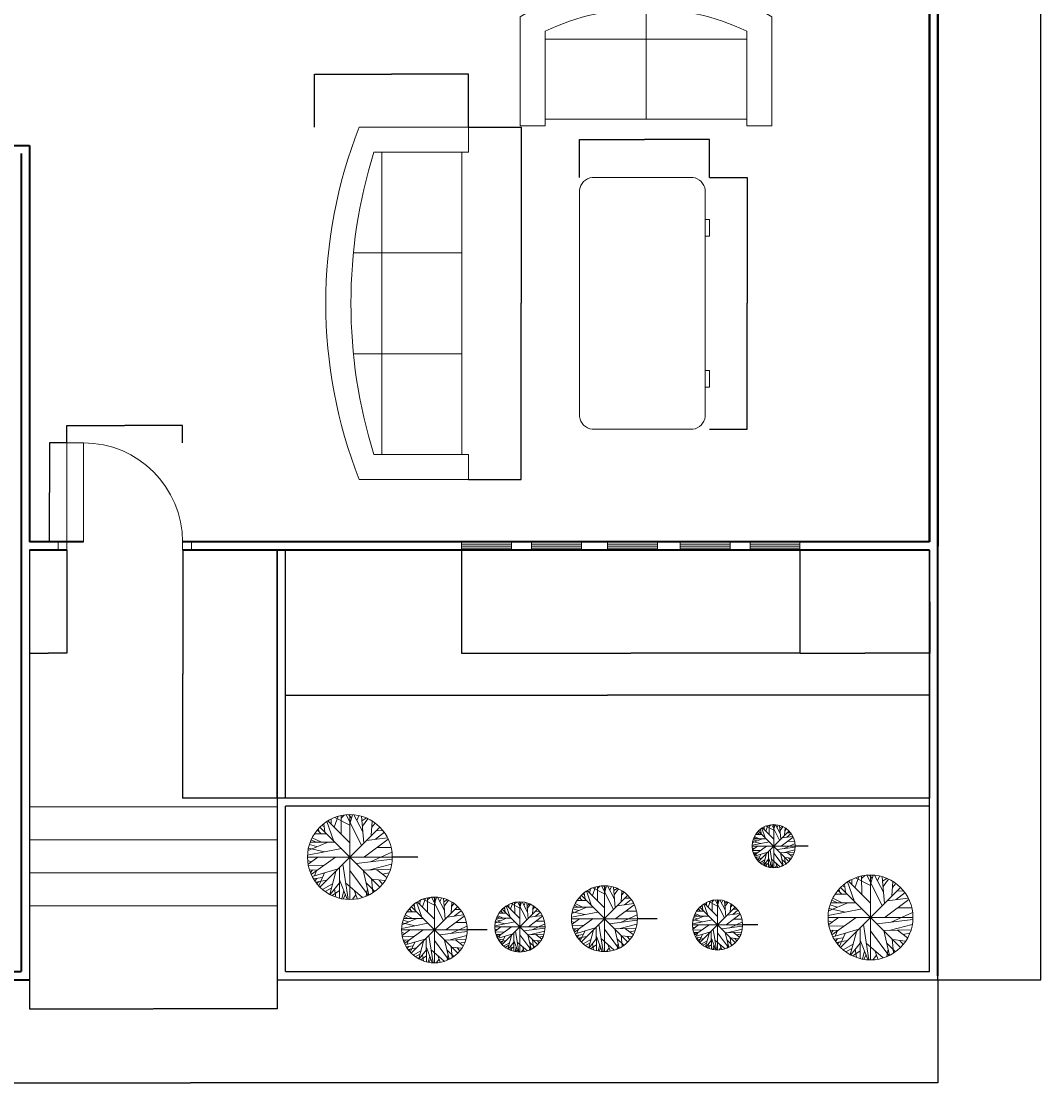
# Model space of a CAD drawing. Units: millimetres. Extents: x 1194 to 22780, y 83 to 13378.
# Tile 1 of 6: x 5317 to 11490, y 83 to 6507. Entities that reach past the tile are written whole.
import ezdxf

# ---------------------------------------------------------------- set-up
doc = ezdxf.new("R2010")
doc.units = ezdxf.units.MM
for name, color, linetype, lineweight in [('A-ANNO-DIMS', 2, 'Continuous', 18), ('A-DOOR', 3, 'Continuous', 18), ('A-FLOR-EDGE', 9, 'Continuous', 25), ('A-FLOR-STRS', 7, 'Continuous', 18), ('A-FURN', 8, 'Continuous', 18), ('A-GLAZ', 4, 'Continuous', 18), ('A-WALL', 7, 'Continuous', 35), ('L-PLNT', 3, 'Continuous', 13)]:
    doc.layers.add(name, color=color, linetype=linetype, lineweight=lineweight)
doc.styles.get("Standard").update_dxf_attribs({"font": 'arial.ttf'})
doc.dimstyles.get("Standard").update_dxf_attribs({"dimtxt": 0.18, "dimasz": 0.18, "dimexe": 0.18, "dimexo": 0.0625, "dimgap": 0.09, "dimtad": 0, "dimtih": 1, "dimtoh": 1, "dimdec": 4, "dimzin": 0, "dimdsep": 46, "dimtxsty": 'Standard', "dimcen": 0.09, "dimadec": 0, "dimazin": 0, "dimtfac": 1, "dimtdec": 4, "dimtofl": 0, "dimtmove": 0, "dimatfit": 3, "dimfxl": 1, "dimtolj": 1, "dimtzin": 0, "dimarcsym": 0})

# ---------------------------------------------------------------- blocks, each defined once
blk = doc.blocks.new('Sofa - Roundback 7 ft.')
for p, q in [((-12.00002, -32.44210000000393), (-12.00003, -6.597100000003898)), ((11.99996999999999, -32.44210000000393), (11.99997999999999, -6.597100000003898)), ((-36.000027, -34.00000000000395), (-36.000027, -11.46960000000396)), ((35.99997999999999, -34.00000000000395), (35.99997999999999, -11.46960000000396)), ((-35.999844, -13.38190000000397), (35.99979999999999, -13.38190000000397)), ((-36.000027, -32.44210000000393), (35.99997999999999, -32.44210000000393))]:
    blk.add_line(p, q)
for points in [[(-36.000027, -34.00000000000395), (-42.000027, -34.00000000000395), (-42.000027, -8.000000000003944)], [(41.99997999999999, -8.000000000003944), (41.99997999999999, -34.00000000000395), (35.99997999999999, -34.00000000000395)]]:
    blk.add_lwpolyline(points)
for centre, radius, start, end in [((0, -114.2500000000039), 114.2500000000039, 68.43141000000072, 111.5686000000006), ((-1.00000000032e-05, -127.1968000000039), 121.1967999999973, 72.72032999999948, 107.2797000000005)]:
    blk.add_arc(centre, radius, start, end)
blk = doc.blocks.new('Sofa - Roundback Loveseat 5 ft.')
for p, q in [((0, -32.44198000000246), (0, -5.999980000002448)), ((-23.99999999999999, -33.99998000000245), (-23.99999999999999, -11.46958000000243)), ((24.00004000000001, -33.99998000000245), (24.00004000000001, -11.46958000000243)), ((-23.99979999999998, -13.38178000000245), (23.99986, -13.38178000000245)), ((-23.99999999999999, -32.44198000000246), (24.00004000000001, -32.44198000000246))]:
    blk.add_line(p, q)
for points in [[(-23.99999999999999, -33.99998000000245), (-29.99999999999999, -33.99998000000245), (-29.99999999999999, -7.999980000002448)], [(30.00004000000001, -7.999980000002448), (30.00004000000001, -33.99998000000245), (24.00004000000001, -33.99998000000245)]]:
    blk.add_lwpolyline(points)
for centre, radius, start, end in [((0, -60.24998000000245), 60.24998000000245, 60.13715000000122, 119.862800000004), ((0, -61.38438000000245), 55.38444000000723, 64.32083000000306, 115.6791999999996)]:
    blk.add_arc(centre, radius, start, end)
blk = doc.blocks.new('Desk - 30 x 60 in.')
for p, q in [((-26.999995, 0), (26.999995, 0)), ((-29.999995, -27), (-29.999995, -3)), ((29.999995, -3), (29.999995, -27)), ((26.999995, -30), (-26.999995, -30)), ((-20.000005, -30), (-20.000005, -31)), ((-16.000005, -31), (-16.000005, -30)), ((15.999995, -31), (15.999995, -30)), ((19.999995, -30), (19.999995, -31)), ((-20.000005, -31), (-16.000005, -31)), ((19.999995, -31), (15.999995, -31))]:
    blk.add_line(p, q)
for centre, radius, start, end in [((-26.499995, -3.5), 3.535534000004229, 98.1300999999916, 171.8698999999352), ((26.499995, -3.5), 3.535533999997753, 8.130102000022115, 81.8698999999439), ((-26.499995, -26.5), 3.535534000000845, 188.1301000000653, 261.8699000000085), ((26.499995, -26.5), 3.535534000004826, 278.1301000000561, 351.8698999999439)]:
    blk.add_arc(centre, radius, start, end)
blk = doc.blocks.new('Window - Wood Frame 36 in. Wide plan')
for p, q in [((0, 6), (0, 0)), ((0, 4.5), (36, 4.5)), ((0, 3), (36, 3)), ((0, 1.5), (36, 1.5)), ((36, 6), (36, 0))]:
    blk.add_line(p, q)
blk = doc.blocks.new('Tree - deciduous plan')
for p, q in [((-37.01069999999993, 47.04079999999987), (-35.25, 35.52979999999991)), ((-32.60919999999999, 50.42639999999995), (-23.27819999999997, 23.56739999999991)), ((-31.20079999999996, 51.10349999999994), (-0.2148999999999432, 20.18179999999984)), ((-26.44719999999995, 46.58939999999984), (-26.27120000000002, 53.81159999999988)), ((-22.04579999999999, 42.07529999999986), (-16.58809999999994, 57.64859999999988)), ((-21.16559999999993, 55.84359999999981), (-0.0387999999999238, 45.00939999999991)), ((-12.53879999999992, 54.94059999999979), (-7.961299999999937, 59.45459999999991)), ((-12.36270000000002, 32.14429999999993), (-12.53879999999992, 58.77760000000001)), ((-5.320499999999924, 59.68059999999979), (16.51049999999998, 16.79629999999986)), ((2.426000000000044, 54.94059999999979), (-1.447199999999952, 59.90559999999982)), ((0, 59.99959999999987), (0, -60.00000000000011)), ((0.4894000000000461, 48.62079999999991), (3.658400000000028, 59.68059999999979)), ((18.27110000000004, 35.52979999999991), (5.418999999999982, 59.68059999999979)), ((9.820299999999975, 51.55489999999986), (12.81330000000002, 58.55159999999989)), ((19.67950000000007, 19.50469999999984), (16.33440000000007, 57.64859999999988)), ((17.03870000000006, 51.10349999999994), (23.20060000000001, 55.16659999999991)), ((17.74290000000007, 43.65519999999992), (25.48940000000005, 54.26359999999988)), ((31.65129999999999, 50.87779999999987), (30.24290000000008, 30.56429999999989)), ((31.1232, 42.52669999999989), (35.87670000000003, 48.16929999999991)), ((-49.86270000000001, 32.82139999999993), (-32.78530000000001, 32.82139999999993)), ((-45.81339999999999, 38.23829999999987), (-40.53179999999997, 33.04709999999989)), ((-43.8768, 36.43259999999998), (-44.40499999999997, 40.26959999999997)), ((42, 41.99999999999988), (-42, -42.00000000000011)), ((42, -42.00000000000011), (-42, 41.99999999999988)), ((-40.17970000000002, 44.55799999999988), (-36.48249999999996, 43.20379999999988)), ((36.22879999999998, 25.14739999999995), (48.90489999999999, 35.07839999999987)), ((37.10910000000001, 37.10979999999995), (46.61609999999996, 37.56119999999987)), ((-32.25709999999992, 20.63329999999985), (-59.19370000000004, 9.347999999999843)), ((-57.08100000000001, 17.92479999999989), (-47.04579999999999, 14.7648999999999)), ((-56.02469999999994, 20.85899999999992), (-20.8134, 20.85899999999992)), ((-54.79229999999995, 24.47019999999986), (-47.75, 21.08469999999988)), ((-53.20780000000002, 27.4043999999999), (-40.17970000000002, 20.85899999999992)), ((54.36260000000004, 25.37309999999991), (20.91190000000006, 0.3197999999998728)), ((23.37670000000003, 23.34169999999994), (53.30629999999996, 27.4043999999999)), ((-59.72190000000001, 2.802499999999895), (-12.01059999999995, 12.05649999999991)), ((-58.66559999999992, 12.73359999999991), (-35.95429999999999, 7.542399999999929)), ((-54.61619999999993, -24.73350000000016), (-20.28530000000001, 0.0940999999999122)), ((29.36260000000004, -6.677100000000109), (59.46820000000002, 7.090999999999894)), ((38.51750000000004, 13.4106999999999), (58.23590000000002, 13.63639999999987)), ((-60, -1.137e-13), (60, -1.137e-13)), ((-59.72190000000001, -4.871400000000107), (-54.26409999999998, -6.677100000000109)), ((-45.2853, -0.1316000000001622), (-59.01769999999999, -10.06270000000006)), ((-58.48950000000002, -12.31970000000012), (-36.48249999999996, -11.64260000000013)), ((-10.07399999999995, -10.06270000000006), (-2.503600000000005, -59.71780000000013)), ((9.29219999999998, -9.159800000000132), (59.64430000000004, -2.84010000000012)), ((26.36969999999997, -18.41380000000015), (58.94010000000003, -9.836900000000128)), ((-57.08100000000001, -18.41380000000015), (-45.2853, -17.9624)), ((-52.67970000000002, -18.1880000000001), (-55.49659999999994, -22.02510000000007)), ((-53.20780000000002, -27.44200000000012), (-16.76409999999998, -16.60810000000015)), ((-38.94719999999995, -29.02190000000008), (-51.44719999999995, -30.60180000000014)), ((-47.2219, -19.31660000000011), (-50.21479999999996, -26.31350000000009)), ((-35.95429999999999, -22.4765000000001), (-44.05290000000002, -40.53290000000015)), ((-19.93309999999997, -20.21940000000018), (-28.55989999999997, -52.72100000000012)), ((-14.82749999999998, -15.02820000000008), (-14.65149999999994, -57.68650000000014)), ((-0.0387999999999238, -19.09090000000015), (25.8415, -53.84950000000015)), ((18.6232, -18.63940000000013), (26.72180000000003, -53.39810000000011)), ((18.79920000000004, -18.63940000000013), (57.35559999999998, -17.28530000000012)), ((38.16539999999998, -18.1880000000001), (52.42600000000004, -29.02190000000008)), ((45.91190000000006, -24.05640000000017), (55.59500000000003, -22.25080000000014)), ((-46.51769999999999, -30.15040000000011), (-49.51059999999995, -33.53600000000006)), ((-32.43309999999997, -32.40750000000014), (-48.10209999999995, -35.56740000000002)), ((-43.70079999999996, -34.66450000000009), (-46.69370000000003, -37.37300000000016)), ((-24.68669999999998, -37.8244000000002), (-38.77120000000002, -45.72410000000013)), ((-26.27120000000002, -43.91850000000011), (-34.72190000000001, -48.65830000000006)), ((-14.65149999999994, -36.24450000000013), (-27.67970000000003, -52.94670000000007)), ((-14.65149999999994, -32.18180000000007), (-3.912000000000034, -59.49220000000014)), ((-6.200799999999958, -36.24450000000013), (17.91899999999998, -57.00940000000014)), ((22.84850000000006, -36.47020000000009), (35.34850000000006, -48.43260000000009)), ((24.78520000000003, -44.82130000000006), (23.02459999999996, -54.97800000000006)), ((30.41899999999998, -30.15040000000011), (32.35559999999998, -50.01250000000016)), ((31.47530000000006, -31.27900000000011), (49.60910000000001, -33.3103000000001)), ((41.51049999999997, -32.6332000000001), (46.08799999999996, -38.05010000000016)), ((-14.65149999999994, -47.30410000000006), (-25.03879999999993, -54.30090000000006)), ((-21.51769999999999, -45.49840000000005), (-19.93309999999997, -56.1065000000001)), ((-8.48950000000002, -47.52980000000014), (-11.48249999999996, -58.58930000000009)), ((-6.376800000000002, -52.72100000000012), (-9.369799999999941, -58.81500000000006)), ((8.41190000000006, -53.17240000000004), (3.834400000000073, -59.49220000000014)), ((5.947099999999977, -46.62690000000009), (10.52459999999996, -58.58930000000009))]:
    blk.add_line(p, q)
blk.add_circle((0, -1.137e-13), 60)
blk = doc.blocks.new('DOOR-SWING-600')
for p, q in [((-0.0004640084134735, -0.0001152583831754), (-0.0004640084134735, 599.9998847416168)), ((-0.0004640084134735, 599.9998847416168), (99.99953599158653, 599.9998847416168)), ((99.99953599158653, 599.9998847416168), (99.99953599158653, -0.0001152583831754))]:
    blk.add_line(p, q)
blk.add_arc((99.99953599158653, -0.0001152583831754), 600, 0, 90)
blk = doc.blocks.new('*D19')
at = {"layer": 'A-ANNO-DIMS', "color": 0, "lineweight": -2, "transparency": 16777216}
for p, q in [((5594.319535991585, 3955.836384741617), (5594.319535991585, 4060.953884741617)), ((5594.499535991586, 4060.773884741617), (5943.313881148475, 4060.773884741617)), ((6294.139535991585, 4060.773884741617), (5945.325190834696, 4060.773884741617)), ((6294.319535991586, 3955.836384741617), (6294.319535991586, 4060.953884741617))]:
    blk.add_line(p, q, dxfattribs=at)
at = {"layer": 'A-ANNO-DIMS', "color": 0, "transparency": 16777216}
for points in [[(5594.499535991586, 4060.803884741616), (5594.499535991586, 4060.743884741617), (5594.319535991585, 4060.773884741617)], [(6294.139535991585, 4060.803884741616), (6294.139535991585, 4060.743884741617), (6294.319535991586, 4060.773884741617)]]:
    blk.add_solid(points, dxfattribs=at)
at = {"layer": 'Defpoints', "color": 0, "transparency": 16777216}
for p in [(6294.319535991586, 4060.773884741617), (5594.319535991585, 3955.773884741617), (6294.319535991586, 3955.773884741617)]:
    blk.add_point(p, dxfattribs=at)
at = {"layer": 'A-ANNO-DIMS', "color": 0, "transparency": 16777216, "insert": (5944.319535991585, 4060.773884741617), "char_height": 0.18, "attachment_point": 5}
blk.add_mtext('\\A1;DOOR 700 TYP.', dxfattribs=at)
blk = doc.blocks.new('*D20')
at = {"layer": 'A-ANNO-DIMS', "color": 0, "lineweight": -2, "transparency": 16777216}
for p, q in [((5594.257035991587, 3955.773884741619), (5489.139535991589, 3955.773884741619)), ((5489.319535991589, 3955.593884741619), (5489.319535991589, 3655.955787879409)), ((5489.319535991589, 3355.953884741619), (5489.319535991589, 3655.591981603829)), ((5594.257035991587, 3355.773884741619), (5489.139535991589, 3355.773884741619))]:
    blk.add_line(p, q, dxfattribs=at)
at = {"layer": 'A-ANNO-DIMS', "color": 0, "transparency": 16777216}
for points in [[(5489.289535991589, 3955.593884741619), (5489.349535991589, 3955.593884741619), (5489.319535991589, 3955.773884741619)], [(5489.289535991589, 3355.953884741619), (5489.349535991589, 3355.953884741619), (5489.319535991589, 3355.773884741619)]]:
    blk.add_solid(points, dxfattribs=at)
at = {"layer": 'Defpoints', "color": 0, "transparency": 16777216}
for p in [(5489.319535991589, 3955.773884741619), (5594.319535991587, 3955.773884741619), (5594.319535991587, 3355.773884741619)]:
    blk.add_point(p, dxfattribs=at)
at = {"layer": 'A-ANNO-DIMS', "color": 0, "transparency": 16777216, "insert": (5489.319535991589, 3655.773884741616), "char_height": 0.18, "attachment_point": 5}
blk.add_mtext('\\A1;600 TYP.', dxfattribs=at)
blk = doc.blocks.new('*D31')
at = {"layer": 'A-ANNO-DIMS', "color": 0, "lineweight": -2, "transparency": 16777216}
for p, q in [((8024.9386296235, 5866.896359479268), (8345.096343171488, 5866.896359479268)), ((8344.91634317149, 5866.716359479267), (8344.91634317149, 4800.279344007587)), ((8344.91634317149, 3733.475943815578), (8344.91634317149, 4799.912959287258)), ((8024.93893202036, 3733.295943815578), (8345.096343171488, 3733.295943815578))]:
    blk.add_line(p, q, dxfattribs=at)
at = {"layer": 'A-ANNO-DIMS', "color": 0, "transparency": 16777216}
for points in [[(8344.886343171485, 5866.716359479267), (8344.946343171488, 5866.716359479267), (8344.91634317149, 5866.896359479268)], [(8344.88634317149, 3733.475943815578), (8344.94634317149, 3733.475943815578), (8344.91634317149, 3733.295943815578)]]:
    blk.add_solid(points, dxfattribs=at)
at = {"layer": 'Defpoints', "color": 0, "transparency": 16777216}
for p in [(8024.8761296235, 5866.896359479268), (8344.91634317149, 5866.896359479268), (8024.876432020361, 3733.295943815578)]:
    blk.add_point(p, dxfattribs=at)
at = {"layer": 'A-ANNO-DIMS', "color": 0, "transparency": 16777216, "insert": (8344.91634317149, 4800.096151647419), "char_height": 0.18, "attachment_point": 5}
blk.add_mtext('\\A1;SOFA 2134 TYP.', dxfattribs=at)
blk = doc.blocks.new('*D32')
at = {"layer": 'A-ANNO-DIMS', "color": 0, "lineweight": -2, "transparency": 16777216}
for p, q in [((7093.54276755999, 5866.958727480659), (7093.542722183807, 6187.116289830213)), ((7093.722722209318, 6186.936289855724), (7558.611388229824, 6186.936355744759)), ((8024.69608426397, 6186.936421803308), (7559.807418243467, 6186.936355914273)), ((8024.876129614641, 5866.958859479268), (8024.876084238458, 6187.116421828821))]:
    blk.add_line(p, q, dxfattribs=at)
at = {"layer": 'A-ANNO-DIMS', "color": 0, "transparency": 16777216}
for points in [[(7093.722722205066, 6186.966289855724), (7093.72272221357, 6186.906289855723), (7093.542722209318, 6186.936289830213)], [(8024.696084259717, 6186.966421803308), (8024.696084268221, 6186.906421803308), (8024.87608426397, 6186.93642182882)]]:
    blk.add_solid(points, dxfattribs=at)
at = {"layer": 'Defpoints', "color": 0, "transparency": 16777216}
for p in [(7093.542722209318, 6186.936289830213), (7093.542767568848, 5866.896227480658), (8024.876129623498, 5866.896359479268)]:
    blk.add_point(p, dxfattribs=at)
at = {"layer": 'A-ANNO-DIMS', "color": 0, "transparency": 16777216, "insert": (7559.209403236645, 6186.936355829516), "char_height": 0.18, "attachment_point": 5}
blk.add_mtext('\\A1;931 TYP.', dxfattribs=at)
blk = doc.blocks.new('*D43')
at = {"layer": 'A-ANNO-DIMS', "color": 0, "lineweight": -2, "transparency": 16777216}
for p, q in [((9484.758350555348, 5562.096129861136), (9713.475813321516, 5562.096129861136)), ((9713.295813321516, 5561.916129861136), (9713.295813321516, 4800.279323551006)), ((9713.29581332152, 4038.276378086716), (9713.295813321516, 4799.913184396845)), ((9484.758350555348, 4038.096378086716), (9713.475813321518, 4038.096378086716))]:
    blk.add_line(p, q, dxfattribs=at)
at = {"layer": 'A-ANNO-DIMS', "color": 0, "transparency": 16777216}
for points in [[(9713.265813321515, 5561.916129861136), (9713.325813321517, 5561.916129861136), (9713.295813321516, 5562.096129861136)], [(9713.265813321517, 4038.276378086716), (9713.325813321519, 4038.276378086716), (9713.29581332152, 4038.096378086716)]]:
    blk.add_solid(points, dxfattribs=at)
at = {"layer": 'Defpoints', "color": 0, "transparency": 16777216}
for p in [(9484.695850555348, 5562.096129861136), (9713.295813321516, 5562.096129861136), (9484.695850555348, 4038.096378086716)]:
    blk.add_point(p, dxfattribs=at)
at = {"layer": 'A-ANNO-DIMS', "color": 0, "transparency": 16777216, "insert": (9713.295813321516, 4800.096253973922), "char_height": 0.18, "attachment_point": 5}
blk.add_mtext('\\A1;DESK 1524', dxfattribs=at)
blk = doc.blocks.new('*D44')
at = {"layer": 'A-ANNO-DIMS', "color": 0, "lineweight": -2, "transparency": 16777216}
for p, q in [((8697.295847668129, 5562.158629861134), (8697.295847668129, 5790.876092627298)), ((8697.475847668127, 5790.696092627298), (9090.707738606961, 5790.696092627298)), ((9484.515850555345, 5790.696092627298), (9091.283959616509, 5790.696092627298)), ((9484.695850555345, 5562.158629861134), (9484.695850555345, 5790.876092627298))]:
    blk.add_line(p, q, dxfattribs=at)
at = {"layer": 'A-ANNO-DIMS', "color": 0, "transparency": 16777216}
for points in [[(8697.475847668127, 5790.726092627298), (8697.475847668127, 5790.666092627298), (8697.295847668129, 5790.696092627298)], [(9484.515850555345, 5790.726092627298), (9484.515850555345, 5790.666092627298), (9484.695850555345, 5790.696092627298)]]:
    blk.add_solid(points, dxfattribs=at)
at = {"layer": 'Defpoints', "color": 0, "transparency": 16777216}
for p in [(8697.295847668129, 5790.696092627298), (8697.295847668129, 5562.096129861135), (9484.695850555345, 5562.096129861135)]:
    blk.add_point(p, dxfattribs=at)
at = {"layer": 'A-ANNO-DIMS', "color": 0, "transparency": 16777216, "insert": (9090.995849111736, 5790.696092627298), "char_height": 0.18, "attachment_point": 5}
blk.add_mtext('\\A1;787', dxfattribs=at)
blk = doc.blocks.new('*D51')
at = {"layer": 'A-ANNO-DIMS', "color": 0, "lineweight": -2, "transparency": 16777216}
for p, q in [((1817.4811, 705.711385), (1817.4811, 83.093885)), ((10867.4811, 705.711385), (10867.4811, 83.093885)), ((1817.6611, 83.273885), (6342.122634788541, 83.273885)), ((10867.3011, 83.273885), (6342.839565211459, 83.273885))]:
    blk.add_line(p, q, dxfattribs=at)
at = {"layer": 'A-ANNO-DIMS', "color": 0, "transparency": 16777216}
for points in [[(1817.6611, 83.30388500000001), (1817.6611, 83.243885), (1817.4811, 83.273885)], [(10867.3011, 83.30388500000001), (10867.3011, 83.243885), (10867.4811, 83.273885)]]:
    blk.add_solid(points, dxfattribs=at)
at = {"layer": 'Defpoints', "color": 0, "transparency": 16777216}
for p in [(1817.4811, 705.773885), (10867.4811, 705.773885), (10867.4811, 83.273885)]:
    blk.add_point(p, dxfattribs=at)
at = {"layer": 'A-ANNO-DIMS', "color": 0, "transparency": 16777216, "insert": (6342.4811, 83.273885), "char_height": 0.18, "attachment_point": 5}
blk.add_mtext('\\A1;9050', dxfattribs=at)
blk = doc.blocks.new('*D52')
at = {"layer": 'A-ANNO-DIMS', "color": 0, "lineweight": -2, "transparency": 16777216}
for p, q in [((10867.5436, 12755.77388500001), (11490.1611, 12755.77388500001)), ((11489.9811, 12755.593885), (11489.98110000001, 6730.955788137794)), ((11489.98110000001, 705.9538850000002), (11489.98110000001, 6730.591981862215)), ((10867.5436, 705.7738850000001), (11490.16110000001, 705.7738850000003))]:
    blk.add_line(p, q, dxfattribs=at)
at = {"layer": 'A-ANNO-DIMS', "color": 0, "transparency": 16777216}
for points in [[(11489.9511, 12755.593885), (11490.01110000001, 12755.593885), (11489.9811, 12755.77388500001)], [(11489.95110000001, 705.9538850000002), (11490.01110000001, 705.9538850000002), (11489.98110000001, 705.7738850000003)]]:
    blk.add_solid(points, dxfattribs=at)
at = {"layer": 'Defpoints', "color": 0, "transparency": 16777216}
for p in [(10867.4811, 12755.77388500001), (11489.9811, 12755.77388500001), (10867.4811, 705.7738850000001)]:
    blk.add_point(p, dxfattribs=at)
at = {"layer": 'A-ANNO-DIMS', "color": 0, "transparency": 16777216, "insert": (11489.98110000001, 6730.773884999999), "char_height": 0.18, "attachment_point": 5}
blk.add_mtext('\\A1;12050', dxfattribs=at)
blk = doc.blocks.new('*D57')
at = {"layer": 'A-ANNO-DIMS', "color": 0, "lineweight": -2, "transparency": 16777216}
for p, q in [((5367.4811, 1152.796637), (5367.4811, 530.1791370000001)), ((6867.4811, 1152.796637), (6867.4811, 530.1791370000001)), ((5367.6611, 530.359137), (6117.131106821283, 530.359137)), ((6867.3011, 530.359137), (6117.831093178717, 530.359137))]:
    blk.add_line(p, q, dxfattribs=at)
at = {"layer": 'A-ANNO-DIMS', "color": 0, "transparency": 16777216}
for points in [[(5367.6611, 530.389137), (5367.6611, 530.3291370000001), (5367.4811, 530.359137)], [(6867.3011, 530.389137), (6867.3011, 530.3291370000001), (6867.4811, 530.359137)]]:
    blk.add_solid(points, dxfattribs=at)
at = {"layer": 'Defpoints', "color": 0, "transparency": 16777216}
for p in [(5367.4811, 1152.859137), (6867.4811, 1152.859137), (5367.4811, 530.359137)]:
    blk.add_point(p, dxfattribs=at)
at = {"layer": 'A-ANNO-DIMS', "color": 0, "transparency": 16777216, "insert": (6117.4811, 530.359137), "char_height": 0.18, "attachment_point": 5}
blk.add_mtext('\\A1;1500', dxfattribs=at)
blk = doc.blocks.new('*D58')
at = {"layer": 'A-ANNO-DIMS', "color": 0, "lineweight": -2, "transparency": 16777216}
for p, q in [((6917.4811, 1805.836385), (6917.4811, 2428.453885)), ((6917.661100000001, 2428.273885), (8867.122696180082, 2428.273885)), ((10817.3011, 2428.273885), (8867.83950381992, 2428.273885)), ((10817.4811, 1805.836385), (10817.4811, 2428.453885))]:
    blk.add_line(p, q, dxfattribs=at)
at = {"layer": 'A-ANNO-DIMS', "color": 0, "transparency": 16777216}
for points in [[(6917.661100000001, 2428.303885), (6917.661100000001, 2428.243885), (6917.4811, 2428.273885)], [(10817.3011, 2428.303885), (10817.3011, 2428.243885), (10817.4811, 2428.273885)]]:
    blk.add_solid(points, dxfattribs=at)
at = {"layer": 'Defpoints', "color": 0, "transparency": 16777216}
for p in [(10817.4811, 2428.273885), (6917.4811, 1805.773885), (10817.4811, 1805.773885)]:
    blk.add_point(p, dxfattribs=at)
at = {"layer": 'A-ANNO-DIMS', "color": 0, "transparency": 16777216, "insert": (8867.4811, 2428.273885), "char_height": 0.18, "attachment_point": 5}
blk.add_mtext('\\A1;3900', dxfattribs=at)
blk = doc.blocks.new('*D62')
at = {"layer": 'A-ANNO-DIMS', "color": 0, "lineweight": -2, "transparency": 16777216}
for p, q in [((6917.418600000003, 3305.773885000002), (6294.801100000007, 3305.773885000002)), ((6294.981100000008, 3305.593885000002), (6294.981100000008, 2555.955788137791)), ((6294.981100000008, 1805.953885000001), (6294.981100000008, 2555.591981862212)), ((6917.418600000003, 1805.773885000001), (6294.801100000007, 1805.773885))]:
    blk.add_line(p, q, dxfattribs=at)
at = {"layer": 'A-ANNO-DIMS', "color": 0, "transparency": 16777216}
for points in [[(6294.951100000008, 3305.593885000002), (6295.011100000007, 3305.593885000002), (6294.981100000008, 3305.773885000002)], [(6294.951100000009, 1805.953885000001), (6295.011100000007, 1805.953885000001), (6294.981100000008, 1805.773885)]]:
    blk.add_solid(points, dxfattribs=at)
at = {"layer": 'Defpoints', "color": 0, "transparency": 16777216}
for p in [(6294.981100000008, 3305.773885000002), (6917.481100000003, 3305.773885000002), (6917.481100000003, 1805.773885000001)]:
    blk.add_point(p, dxfattribs=at)
at = {"layer": 'A-ANNO-DIMS', "color": 0, "transparency": 16777216, "insert": (6294.981100000007, 2555.773884999999), "char_height": 0.18, "attachment_point": 5}
blk.add_mtext('\\A1;1500', dxfattribs=at)
blk = doc.blocks.new('*D67')
at = {"layer": 'A-ANNO-DIMS', "color": 0, "lineweight": -2, "transparency": 16777216}
for p, q in [((7983.786704999999, 3305.383366), (7983.786704999999, 2682.765866)), ((10032.104138, 3305.383366), (10032.104138, 2682.765866)), ((7983.966705, 2682.945866), (9007.480257789222, 2682.945866)), ((10031.924138, 2682.945866), (9008.410585210779, 2682.945866))]:
    blk.add_line(p, q, dxfattribs=at)
at = {"layer": 'A-ANNO-DIMS', "color": 0, "transparency": 16777216}
for points in [[(7983.966705, 2682.975866), (7983.966705, 2682.915866), (7983.786704999999, 2682.945866)], [(10031.924138, 2682.975866), (10031.924138, 2682.915866), (10032.104138, 2682.945866)]]:
    blk.add_solid(points, dxfattribs=at)
at = {"layer": 'Defpoints', "color": 0, "transparency": 16777216}
for p in [(7983.786704999999, 3305.445866), (10032.104138, 3305.445866), (7983.786704999999, 2682.945866)]:
    blk.add_point(p, dxfattribs=at)
at = {"layer": 'A-ANNO-DIMS', "color": 0, "transparency": 16777216, "insert": (9007.945421500002, 2682.945866), "char_height": 0.18, "attachment_point": 5}
blk.add_mtext('\\A1;2048.3', dxfattribs=at)
blk = doc.blocks.new('*D68')
at = {"layer": 'A-ANNO-DIMS', "color": 0, "lineweight": -2, "transparency": 16777216}
for p, q in [((10032.10416410359, 3305.383366005452), (10032.3642049862, 2682.765920703064)), ((10817.4811261036, 3305.711385005452), (10817.74116698636, 2683.093939328176)), ((10032.54412979215, 2682.945995865719), (10424.66001189933, 2683.109766028019)), ((10817.56109182371, 2683.273864134122), (10425.44520971652, 2683.110093971823))]:
    blk.add_line(p, q, dxfattribs=at)
at = {"layer": 'A-ANNO-DIMS', "color": 0, "transparency": 16777216}
for points in [[(10032.54411726242, 2682.975995863102), (10032.54414232187, 2682.915995868335), (10032.36412980785, 2682.945920687365)], [(10817.56107929398, 2683.303864131506), (10817.56110435343, 2683.243864136739), (10817.74109180801, 2683.273939312477)]]:
    blk.add_solid(points, dxfattribs=at)
at = {"layer": 'Defpoints', "color": 0, "transparency": 16777216}
for p in [(10032.104138, 3305.445866000001), (10817.4811, 3305.773885000001), (10032.36412980785, 2682.945920687365)]:
    blk.add_point(p, dxfattribs=at)
at = {"layer": 'A-ANNO-DIMS', "color": 0, "transparency": 16777216, "insert": (10425.05261080792, 2683.109929999921), "char_height": 0.18, "attachment_point": 5}
blk.add_mtext('\\A1;785.4', dxfattribs=at)
blk = doc.blocks.new('*D69')
at = {"layer": 'A-ANNO-DIMS', "color": 0, "lineweight": -2, "transparency": 16777216}
for p, q in [((5367.4811, 3305.711385), (5367.4811, 2683.093885)), ((5594.319536, 3305.711385), (5594.319536, 2683.093885)), ((5367.6611, 2683.273885), (5480.435522638472, 2683.273885)), ((5594.139536, 2683.273885), (5481.365113361528, 2683.273885))]:
    blk.add_line(p, q, dxfattribs=at)
at = {"layer": 'A-ANNO-DIMS', "color": 0, "transparency": 16777216}
for points in [[(5367.6611, 2683.303885000001), (5367.6611, 2683.243885), (5367.4811, 2683.273885)], [(5594.139536, 2683.303885000001), (5594.139536, 2683.243885), (5594.319536, 2683.273885)]]:
    blk.add_solid(points, dxfattribs=at)
at = {"layer": 'Defpoints', "color": 0, "transparency": 16777216}
for p in [(5367.4811, 3305.773885), (5594.319536, 3305.773885), (5367.4811, 2683.273885)]:
    blk.add_point(p, dxfattribs=at)
at = {"layer": 'A-ANNO-DIMS', "color": 0, "transparency": 16777216, "insert": (5480.900317999999, 2683.273885), "char_height": 0.18, "attachment_point": 5}
blk.add_mtext('\\A1;226.84', dxfattribs=at)
blk = doc.blocks.new('*D94')
at = {"layer": 'A-ANNO-DIMS', "color": 0, "lineweight": -2, "transparency": 16777216}
for p, q in [((7307.195641999998, 1448.826718), (7307.375642, 1448.826717999999)), ((7307.285641999998, 1448.736718), (7307.285641999998, 1448.916717999999)), ((7718.239941199906, 1448.8271692), (7564.312078999998, 1448.827000197628))]:
    blk.add_line(p, q, dxfattribs=at)
at = {"layer": 'A-ANNO-DIMS', "color": 0, "transparency": 16777216}
blk.add_solid([(7564.312078967062, 1448.857000197628), (7564.312079032936, 1448.797000197628), (7564.132078999998, 1448.827)], dxfattribs=at)
at = {"layer": 'Defpoints', "color": 0, "transparency": 16777216}
for p in [(7050.439205, 1448.826436), (7564.132078999998, 1448.827)]:
    blk.add_point(p, dxfattribs=at)
at = {"layer": 'A-ANNO-DIMS', "color": 0, "transparency": 16777216, "insert": (7718.921694269482, 1448.8271692), "char_height": 0.18, "attachment_point": 5}
blk.add_mtext('\\A1;2X ∅513.7', dxfattribs=at)
blk = doc.blocks.new('*D95')
at = {"layer": 'A-ANNO-DIMS', "color": 0, "lineweight": -2, "transparency": 16777216}
for p, q in [((8848.506493, 1076.128227999999), (8848.686492999996, 1076.128227999999)), ((8848.596493, 1076.038228), (8848.596493, 1076.218227999999)), ((9167.969441799922, 1076.127863199999), (9048.384586, 1076.127999794396))]:
    blk.add_line(p, q, dxfattribs=at)
at = {"layer": 'A-ANNO-DIMS', "color": 0, "transparency": 16777216}
blk.add_solid([(9048.384586034268, 1076.157999794396), (9048.384585965732, 1076.097999794396), (9048.204586, 1076.127999999999)], dxfattribs=at)
at = {"layer": 'Defpoints', "color": 0, "transparency": 16777216}
for p in [(8648.988399999995, 1076.128455999999), (9048.204586, 1076.127999999999)]:
    blk.add_point(p, dxfattribs=at)
at = {"layer": 'A-ANNO-DIMS', "color": 0, "transparency": 16777216, "insert": (9168.460144392013, 1076.127863199999), "char_height": 0.18, "attachment_point": 5}
blk.add_mtext('\\A1;∅399.2', dxfattribs=at)
blk = doc.blocks.new('*D96')
at = {"layer": 'A-ANNO-DIMS', "color": 0, "lineweight": -2, "transparency": 16777216}
for p, q in [((7819.127702999998, 1007.942615), (7819.307702999999, 1007.942615)), ((7819.217702999999, 1007.852615), (7819.217702999999, 1008.032615)), ((8137.805598999776, 1007.943231), (8018.515138000001, 1007.943000348035))]:
    blk.add_line(p, q, dxfattribs=at)
at = {"layer": 'A-ANNO-DIMS', "color": 0, "transparency": 16777216}
blk.add_solid([(8018.515137941994, 1007.973000348036), (8018.515138058008, 1007.913000348036), (8018.335138000001, 1007.943)], dxfattribs=at)
at = {"layer": 'Defpoints', "color": 0, "transparency": 16777216}
for p in [(7620.100267999998, 1007.94223), (8018.335138000001, 1007.943)]:
    blk.add_point(p, dxfattribs=at)
at = {"layer": 'A-ANNO-DIMS', "color": 0, "transparency": 16777216, "insert": (8138.296301591863, 1007.943231), "char_height": 0.18, "attachment_point": 5}
blk.add_mtext('\\A1;∅398.2', dxfattribs=at)
blk = doc.blocks.new('*D97')
at = {"layer": 'A-ANNO-DIMS', "color": 0, "lineweight": -2, "transparency": 16777216}
for p, q in [((9533.006967999992, 1038.522900999999), (9533.186967999996, 1038.522900999999)), ((9533.096967999993, 1038.432900999999), (9533.096967999996, 1038.612900999999)), ((9776.606814399982, 1038.523059399999), (9685.470621999995, 1038.523000117087))]:
    blk.add_line(p, q, dxfattribs=at)
at = {"layer": 'A-ANNO-DIMS', "color": 0, "transparency": 16777216}
blk.add_solid([(9685.470621980481, 1038.553000117087), (9685.470622019511, 1038.493000117087), (9685.290621999997, 1038.522999999999)], dxfattribs=at)
at = {"layer": 'Defpoints', "color": 0, "transparency": 16777216}
for p in [(9380.903314, 1038.522801999999), (9685.290621999997, 1038.522999999999)]:
    blk.add_point(p, dxfattribs=at)
at = {"layer": 'A-ANNO-DIMS', "color": 0, "transparency": 16777216, "insert": (9777.288199120308, 1038.523059399999), "char_height": 0.18, "attachment_point": 5}
blk.add_mtext('\\A1;2X ∅304.4', dxfattribs=at)
blk = doc.blocks.new('*D98')
at = {"layer": 'A-ANNO-DIMS', "color": 0, "lineweight": -2, "transparency": 16777216}
for p, q in [((9873.278623999997, 1514.591687), (9873.458624, 1514.591687)), ((9873.368624, 1514.501687), (9873.368624, 1514.681687)), ((10082.61649599977, 1514.5921878), (10004.32854399999, 1514.5920004308))]:
    blk.add_line(p, q, dxfattribs=at)
at = {"layer": 'A-ANNO-DIMS', "color": 0, "transparency": 16777216}
blk.add_solid([(10004.3285439282, 1514.6220004308), (10004.3285440718, 1514.5620004308), (10004.14854399999, 1514.592)], dxfattribs=at)
at = {"layer": 'Defpoints', "color": 0, "transparency": 16777216}
for p in [(9742.588704, 1514.591374), (10004.14854399999, 1514.592)]:
    blk.add_point(p, dxfattribs=at)
at = {"layer": 'A-ANNO-DIMS', "color": 0, "transparency": 16777216, "insert": (10083.17798303934, 1514.5921878), "char_height": 0.18, "attachment_point": 5}
blk.add_mtext('\\A1;∅261.56', dxfattribs=at)

msp = doc.modelspace()

# ---------------------------------------------------------------- linework, layer by layer
at = {"layer": 'A-DOOR'}
for p, q in [((5540.634663159901, 3355.773884741617), (5540.634663159901, 3305.773884741618)), ((5594.319535991586, 3305.773884741618), (5594.319535991586, 3355.773884741617)), ((6294.319535991586, 3355.773884741617), (6294.319535991586, 3305.773884741618)), ((6348.004408823271, 3305.773884741618), (6348.004408823271, 3355.773884741617)), ((5540.634663159901, 3305.773884741618), (5594.319535991586, 3305.773884741618)), ((6294.319535991586, 3305.773884741618), (6348.004408823271, 3305.773884741618))]:
    msp.add_line(p, q, dxfattribs=at)
at = {"layer": 'A-FLOR-EDGE'}
for p, q in [((5367.481100020039, 3305.773884741618), (5367.481100020039, 755.7738847416167)), ((6867.481100020039, 1805.773884741617), (6867.481100020039, 3305.773884741618)), ((6867.481100020039, 3305.773884741618), (6867.481100020039, 755.7738847416166)), ((6917.481100020039, 1805.773884741617), (6917.481100020039, 3305.773884741618)), ((10817.48110002004, 755.7738847416167), (10817.48110002004, 3305.773884741618)), ((10817.48110002004, 3305.773884741618), (10817.48110002004, 1805.773884741617)), ((10817.48110002004, 1805.773884741617), (6917.481100020039, 1805.773884741617)), ((6917.481100020039, 755.7738847416167), (6917.481100020039, 1756.803666472503)), ((10817.48110002004, 1756.803666472503), (6917.481100020039, 1756.803666472503)), ((5367.481100020039, 755.7738847416167), (5367.481100020039, 705.7738847416167)), ((6867.481100020039, 755.7738847416166), (6867.481100020039, 705.7738847416167)), ((6917.48110002004, 755.7738847416167), (10817.48110002004, 755.7738847416167)), ((10867.48110002004, 705.7738847416167), (10867.48110002004, 730.7738847416167)), ((6867.481100020039, 705.7738847416167), (10842.48110002004, 705.7738847416167)), ((10842.48110002004, 705.7738847416167), (10867.48110002004, 705.7738847416167))]:
    msp.add_line(p, q, dxfattribs=at)
at = {"layer": 'A-FLOR-STRS'}
for p, q in [((6867.481100020039, 1752.859137466366), (5367.481100020039, 1752.859137466366)), ((6867.481100020039, 1552.859137466366), (5367.481100020039, 1552.859137466366)), ((6867.481100020039, 1352.859137466366), (5367.481100020039, 1352.859137466366)), ((6867.481100020039, 1152.859137466366), (5367.481100020039, 1152.859137466366))]:
    msp.add_line(p, q, dxfattribs=at)
at = {"layer": 'A-WALL'}
for p, q in [((10867.48110002004, 730.7738847416167), (10867.48110002004, 12730.77388474161)), ((10817.48110002004, 3355.773884741618), (10817.48110002003, 10005.77388474161)), ((10817.48110002004, 6930.773884741618), (10817.48110002004, 3355.773884741618)), ((10867.48110002004, 6930.773884741618), (10867.48110002004, 3330.773884741617)), ((4842.481100020041, 5755.773884741617), (5317.481100020039, 5755.773884741617)), ((5317.48110002004, 5755.773884741617), (5367.481100020039, 5755.773884741617)), ((5367.481100020039, 5755.773884741617), (5367.481100020039, 3355.773884741618)), ((5317.481100020039, 5705.773884741616), (5317.481100020039, 755.7738847416167)), ((5694.319535991586, 3355.773884741618), (5367.481100020039, 3355.773884741617)), ((6642.481100020041, 3355.773884741618), (6294.319535991586, 3355.773884741618)), ((10817.48110002004, 3355.773884741618), (6642.481100020041, 3355.773884741618)), ((5594.319535991586, 3305.773884741618), (5367.481100020039, 3305.773884741618)), ((6642.481100020041, 3305.773884741618), (6294.319535991586, 3305.773884741618)), ((10817.48110002004, 3305.773884741618), (6642.481100020041, 3305.773884741618)), ((1867.481100020041, 755.7738847416167), (5317.481100020039, 755.7738847416167)), ((1842.481100020041, 705.7738847416167), (5367.481100020039, 705.7738847416167))]:
    msp.add_line(p, q, dxfattribs=at)

# ---------------------------------------------------------------- block references
at = {"layer": 'A-DOOR'}
msp.add_blockref('DOOR-SWING-600', (5594.319999999999, 3355.774), dxfattribs=at)
at = {"layer": 'A-FURN', "xscale": 25.4, "yscale": 25.4, "zscale": 25.4}
msp.add_blockref('Sofa - Roundback Loveseat 5 ft.', (9100.229622168534, 6737.50369569763), dxfattribs=at)
at = {"layer": 'A-FURN'}
for name, p, xscale, yscale, zscale, rotation in [('Sofa - Roundback 7 ft.', (7161.276280821768, 4800.096507216861), 25.40000000000001, 25.40000000000001, 25.40000000000001, 90.00000812057576), ('Desk - 30 x 60 in.', (8697.295850555345, 4800.096253973917), 25.4, 25.4, 25.4, 90)]:
    msp.add_blockref(name, p, dxfattribs=dict(at, xscale=xscale, yscale=yscale, zscale=zscale, rotation=rotation))
at = {"layer": 'A-GLAZ', "xscale": 8.388003104210137, "yscale": 8.388003104210137, "zscale": 8.388003104210137}
for p in [(7983.786704636485, 3305.445866116355), (8407.05220250973, 3305.445866116355), (8867.056161980627, 3305.445866116355), (9307.16972035305, 3305.445866116355), (9730.136025906571, 3305.445866116355)]:
    msp.add_blockref('Window - Wood Frame 36 in. Wide plan', p, dxfattribs=at)
at = {"layer": 'L-PLNT'}
for p, xscale, yscale, zscale in [((7307.285642102589, 1448.826717752093), 4.280773954571369, 4.280773954571369, 4.280773954571369), ((9873.368624121817, 1514.591687384594), 2.179665335052035, 2.179665335052035, 2.179665335052035), ((10459.50587753888, 1083.54455620757), 4.280773954571369, 4.280773954571369, 4.280773954571369), ((8848.596492666955, 1076.12822783105), 3.326801558127637, 3.326801558127637, 3.326801558127637), ((7819.217703361866, 1007.942615499665), 3.318623918633804, 3.318623918633804, 3.318623918633804), ((8336.615015703232, 1026.205151581362), 2.536560892470606, 2.536560892470606, 2.536560892470606), ((9533.096968171463, 1038.522901368152), 2.536560892470606, 2.536560892470606, 2.536560892470606)]:
    msp.add_blockref('Tree - deciduous plan', p, dxfattribs=dict(at, xscale=xscale, yscale=yscale, zscale=zscale))

# ---------------------------------------------------------------- dimensions: what is measured, and where the dimension line sits
at = {"layer": 'A-ANNO-DIMS'}
for base, p1, p2, angle, override, picture, middle in [((11489.9811, 12755.77388500001), (10867.4811, 705.773885), (10867.4811, 12755.773885), 90, {"dimdec": 0, "dimlfac": 1, "dimrnd": 0, "dimzin": 0, "dimdsep": 46, "dimlunit": 2}, '*D52', (11489.98110000001, 6730.773884999999)), ((8697.295847668129, 5790.696092627298), (9484.695850555345, 5562.096129861135), (8697.295847668129, 5562.096129861135), 180, {"dimdec": 0, "dimlfac": 1, "dimrnd": 0, "dimzin": 0, "dimdsep": 46, "dimlunit": 2}, '*D44', (9090.995849111736, 5790.696092627298)), ((5367.4811, 2683.273885), (5594.319536, 3305.773885), (5367.4811, 3305.773885), 180, {"dimdec": 2, "dimlfac": 1, "dimrnd": 0, "dimzin": 0, "dimdsep": 46, "dimlunit": 2}, '*D69', (5480.900317999999, 2683.273885)), ((6294.981100000008, 3305.773885000002), (6917.4811, 1805.773885), (6917.4811, 3305.773885), 90, {"dimdec": 0, "dimlfac": 1, "dimrnd": 0, "dimzin": 0, "dimdsep": 46, "dimlunit": 2}, '*D62', (6294.981100000007, 2555.773884999999)), ((7983.786704999999, 2682.945866), (10032.104138, 3305.445866), (7983.786704999999, 3305.445866), 180, {"dimdec": 1, "dimlfac": 1, "dimrnd": 0, "dimzin": 0, "dimdsep": 46, "dimlunit": 2}, '*D67', (9007.945421500002, 2682.945866)), ((10032.36412980785, 2682.945920687365), (10817.4811, 3305.773885), (10032.104138, 3305.445866), 180.0239300140405, {"dimdec": 1, "dimlfac": 1, "dimrnd": 0, "dimzin": 0, "dimdsep": 46, "dimlunit": 2}, '*D68', (10425.05261080792, 2683.109929999921)), ((5367.4811, 530.359137), (6867.4811, 1152.859137), (5367.4811, 1152.859137), 180, {"dimdec": 0, "dimlfac": 1, "dimrnd": 0, "dimzin": 0, "dimdsep": 46, "dimlunit": 2}, '*D57', (6117.4811, 530.359137))]:
    dim = msp.add_linear_dim(base=base, p1=p1, p2=p2, angle=angle, dimstyle='Standard', override=override, dxfattribs=at)
    dim.commit()
    dim.dimension.update_dxf_attribs({"geometry": picture, "text_midpoint": middle})
for base, p1, p2, angle, text, picture, middle in [((7093.542722209318, 6186.936289830213), (8024.876129623498, 5866.896359479266), (7093.542767568847, 5866.896227480658), 180.0000081205757, '<> TYP.', '*D32', (7559.209403236645, 6186.936355829516)), ((8344.91634317149, 5866.896359479268), (8024.876432020358, 3733.295943815576), (8024.876129623498, 5866.896359479266), 90.00000812057576, 'SOFA <> TYP.', '*D31', (8344.91634317149, 4800.096151647419)), ((9713.295813321516, 5562.096129861136), (9484.695850555345, 4038.096378086715), (9484.695850555345, 5562.096129861135), 90, 'DESK <>', '*D43', (9713.295813321516, 4800.096253973922)), ((5489.319535991589, 3955.773884741619), (5594.319535991585, 3355.773884741617), (5594.319535991585, 3955.773884741617), 90, '<> TYP.', '*D20', (5489.319535991589, 3655.773884741616))]:
    dim = msp.add_linear_dim(base=base, p1=p1, p2=p2, angle=angle, text=text, dimstyle='Standard', override={"dimdec": 0, "dimlfac": 1, "dimrnd": 0, "dimzin": 0, "dimdsep": 46, "dimlunit": 2}, dxfattribs=at)
    dim.commit()
    dim.dimension.update_dxf_attribs({"geometry": picture, "text_midpoint": middle})
dim = msp.add_linear_dim(base=(6294.319535991586, 4060.773884741617), p1=(5594.319535991585, 3955.773884741617), p2=(6294.319535991586, 3955.773884741617), text='DOOR <> TYP.', dimstyle='Standard', override={"dimdec": 0, "dimlfac": 1, "dimrnd": 0, "dimzin": 0, "dimdsep": 46, "dimlunit": 2}, dxfattribs=at)
dim.commit()
dim.dimension.update_dxf_attribs({"geometry": '*D19', "text_midpoint": (5944.319535991585, 4060.773884741617)})
for base, p1, p2, picture, middle in [((10817.4811, 2428.273885), (6917.4811, 1805.773885), (10817.4811, 1805.773885), '*D58', (8867.4811, 2428.273885)), ((10867.4811, 83.273885), (1817.4811, 705.773885), (10867.4811, 705.773885), '*D51', (6342.4811, 83.273885))]:
    dim = msp.add_linear_dim(base=base, p1=p1, p2=p2, dimstyle='Standard', override={"dimdec": 0, "dimlfac": 1, "dimrnd": 0, "dimzin": 0, "dimdsep": 46, "dimlunit": 2}, dxfattribs=at)
    dim.commit()
    dim.dimension.update_dxf_attribs({"geometry": picture, "text_midpoint": middle})
for p1, p2, override, picture, middle in [((9742.588704, 1514.591374), (10004.14854399999, 1514.592), {"dimdec": 2, "dimlfac": 1, "dimrnd": 0, "dimzin": 0, "dimdsep": 46, "dimlunit": 2}, '*D98', (10082.61649599977, 1514.5921878)), ((8648.988399999995, 1076.128455999999), (9048.204586, 1076.127999999999), {"dimdec": 1, "dimlfac": 1, "dimrnd": 0, "dimzin": 0, "dimdsep": 46, "dimlunit": 2}, '*D95', (9167.969441799922, 1076.127863199999)), ((7620.100267999998, 1007.94223), (8018.335138000001, 1007.943), {"dimdec": 1, "dimlfac": 1, "dimrnd": 0, "dimzin": 0, "dimdsep": 46, "dimlunit": 2}, '*D96', (8137.805598999776, 1007.943231))]:
    dim = msp.add_diameter_dim_2p(p1=p1, p2=p2, dimstyle='Standard', override=override, dxfattribs=at)
    dim.commit()
    dim.dimension.update_dxf_attribs({"geometry": picture, "text_midpoint": middle, "dimtype": 163})
for p1, p2, picture, middle in [((7050.439205, 1448.826436), (7564.132078999998, 1448.827), '*D94', (7718.239941199906, 1448.8271692)), ((9380.903314, 1038.522801999999), (9685.290621999997, 1038.522999999999), '*D97', (9776.606814399982, 1038.523059399999))]:
    dim = msp.add_diameter_dim_2p(p1=p1, p2=p2, text='2X <>', dimstyle='Standard', override={"dimdec": 1, "dimlfac": 1, "dimrnd": 0, "dimzin": 0, "dimdsep": 46, "dimlunit": 2}, dxfattribs=at)
    dim.commit()
    dim.dimension.update_dxf_attribs({"geometry": picture, "text_midpoint": middle, "dimtype": 163})

doc.saveas('drawing.dxf')
